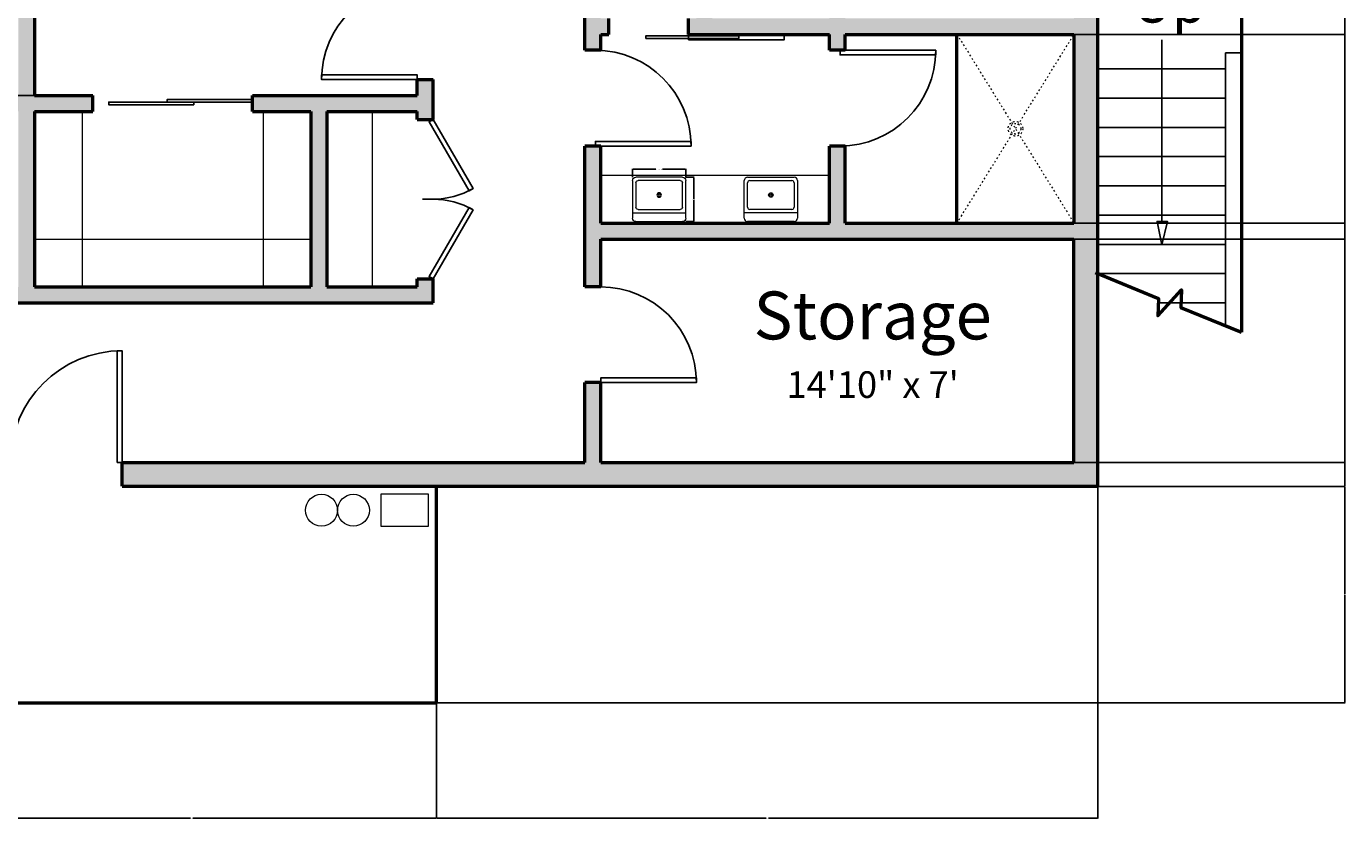
# Model space of a CAD drawing. Units: inches. Extents: x 296 to 2116, y 330 to 1460.
# Tile 8 of 9: x 1620 to 2116, y 779 to 1077. Entities that reach past the tile are written whole.
import ezdxf

# ---------------------------------------------------------------- set-up
doc = ezdxf.new("R2010")
doc.units = ezdxf.units.IN
doc.linetypes.add('ACAD_ISO03W100', pattern=[30, 12, -18])
for name, color, linetype, lineweight in [('A-ANNO-DIMS', 2, 'Continuous', 18), ('A-ANNO-TEXT', 7, 'Continuous', 18), ('A-AREA-IDEN', 7, 'Continuous', 25), ('A-DOOR', 3, 'Continuous', 25), ('A-FLOR-FIXT', 8, 'Continuous', 18), ('A-FLOR-OVHD', 132, 'ACAD_ISO03W100', 18), ('A-FLOR-STRS', 40, 'Continuous', 25), ('A-WALL', 7, 'Continuous', 50), ('A-WALL-PATT', 8, 'Continuous', 13)]:
    doc.layers.add(name, color=color, linetype=linetype, lineweight=lineweight)
doc.styles.add('ATTR', font='romans.shx', dxfattribs={"width": 0.8, "height": 1.075})
doc.styles.get("Standard").update_dxf_attribs({"font": 'arial.ttf'})
doc.dimstyles.get("Standard").update_dxf_attribs({"dimtxt": 0.18, "dimasz": 0.18, "dimexe": 0.18, "dimexo": 0.0625, "dimgap": 0.09, "dimtad": 0, "dimtih": 1, "dimtoh": 1, "dimdec": 4, "dimzin": 0, "dimdsep": 46, "dimtxsty": 'Standard', "dimcen": 0.09, "dimadec": 0, "dimazin": 0, "dimtfac": 1, "dimtdec": 4, "dimtofl": 0, "dimtmove": 0, "dimatfit": 3, "dimfxl": 1, "dimtolj": 1, "dimtzin": 0, "dimarcsym": 0})

# ---------------------------------------------------------------- blocks, each defined once
blk = doc.blocks.new('*U18')
for p, q in [((0, 0), (0, 4)), ((36, 0), (36, 4))]:
    blk.add_line(p, q)
blk.add_lwpolyline([(0, 0), (0, -36), (1.75, -36), (1.75, 0)], close=True)
blk.add_arc((0, 0), 36, 270, 0)
blk = doc.blocks.new('*U19')
for p, q in [((0, 0), (0, -4)), ((36, 0), (36, -4))]:
    blk.add_line(p, q)
blk.add_lwpolyline([(0, 0), (0, 36), (1.75, 36), (1.75, 0)], close=True)
blk.add_arc((0, 0), 36, 0, 90)
blk = doc.blocks.new('*U23')
for p, q in [((-40, 0), (-40, -4)), ((0, 0), (0, -4))]:
    blk.add_line(p, q)
blk.add_lwpolyline([(0, 0), (0, 40), (-1.75, 40), (-1.75, 0)], close=True)
blk.add_arc((0, 0), 40, 90, 180)
blk = doc.blocks.new('*U24')
for p, q in [((0, 0), (0, 4)), ((36, 0), (36, 4))]:
    blk.add_line(p, q)
blk.add_lwpolyline([(0, 0), (0, -36), (1.75, -36), (1.75, 0)], close=True)
blk.add_arc((0, 0), 36, 270, 0)
blk = doc.blocks.new('*U25')
for p, q in [((-36, 0), (-36, 4)), ((0, 0), (0, 4))]:
    blk.add_line(p, q)
blk.add_lwpolyline([(0, 0), (0, -36), (-1.75, -36), (-1.75, 0)], close=True)
blk.add_arc((0, 0), 36, 180, 270)
blk = doc.blocks.new('*U26')
for p, q in [((-30, 0), (-30, 4)), ((0, 0), (0, 4))]:
    blk.add_line(p, q)
blk.add_lwpolyline([(0, 0), (-25.98, -15), (-26.86, -13.48), (-0.88, 1.52)], close=True)
blk.add_arc((0, 0), 30, 180, 210)
blk = doc.blocks.new("24'' Sink Single PV")
blk.add_line((-12.00001, -3.999996), (12, -3.999996))
for points in [[(-10.5, 0), (10.5, 0)], [(-12.00001, -18.499996), (-12.00001, -1.5)], [(-9.5, -5.499996), (9.5, -5.499996)], [(12, -1.5), (12, -18.499996)], [(-10.5, -17.499996), (-10.5, -6.499996)], [(10.5, -6.499996), (10.5, -17.499996)], [(10.5, -19.999996), (-10.5, -19.999996)], [(9.5, -18.499996), (-9.5, -18.499996)]]:
    blk.add_lwpolyline(points)
for radius in [1, 0.5]:
    blk.add_circle((0, -11.999996), radius)
for centre, radius, start, end in [((-10.5, -1.5), 1.5, 90, 180), ((-9.5, -6.499996), 1, 90, 180), ((9.5, -6.499996), 1, 0, 90), ((10.5, -1.5), 1.5, 0, 90), ((-9.5, -17.499996), 1, 180, 270), ((9.5, -17.499996), 1, 270, 0), ((-10.5, -18.499996), 1.5, 180, 270), ((10.5, -18.499996), 1.5, 270, 0)]:
    blk.add_arc(centre, radius, start, end)
at = {"style": 'ATTR', "width": 0.8, "flags": 9}
blk.add_attdef('ESTCODE', (0, 0), '', height=0.0048, dxfattribs=at)
blk = doc.blocks.new('*D37')
at = {"layer": 'A-ANNO-DIMS', "color": 0, "lineweight": -2, "transparency": 16777216}
for p, q in [((1848.18, 1020.25), (1848.18, 1023.37)), ((1848.36, 1023.19), (1856.96, 1023.19)), ((1868, 1023.19), (1859.41, 1023.19)), ((1868.18, 1020.25), (1868.18, 1023.37))]:
    blk.add_line(p, q, dxfattribs=at)
at = {"layer": 'A-ANNO-DIMS', "color": 0, "transparency": 16777216}
for points in [[(1848.36, 1023.22), (1848.36, 1023.16), (1848.18, 1023.19)], [(1868, 1023.22), (1868, 1023.16), (1868.18, 1023.19)]]:
    blk.add_solid(points, dxfattribs=at)
at = {"layer": 'Defpoints', "color": 0, "transparency": 16777216}
for p in [(1868.18, 1023.19), (1848.18, 1020.19), (1868.18, 1020.19)]:
    blk.add_point(p, dxfattribs=at)
at = {"layer": 'A-ANNO-DIMS', "color": 0, "transparency": 16777216, "insert": (1858.18, 1023.19), "char_height": 0.18, "attachment_point": 5}
blk.add_mtext('\\A1;BATH SINK 20 TYP.', dxfattribs=at)
blk = doc.blocks.new('*D38')
at = {"layer": 'A-ANNO-DIMS', "color": 0, "lineweight": -2, "transparency": 16777216}
for p, q in [((1868.25, 1020.19), (1871.36, 1020.19)), ((1871.18, 1020.01), (1871.18, 1012.03)), ((1871.18, 1003.7), (1871.18, 1011.67)), ((1868.25, 1003.52), (1871.36, 1003.52))]:
    blk.add_line(p, q, dxfattribs=at)
at = {"layer": 'A-ANNO-DIMS', "color": 0, "transparency": 16777216}
for points in [[(1871.15, 1020.01), (1871.21, 1020.01), (1871.18, 1020.19)], [(1871.15, 1003.7), (1871.21, 1003.7), (1871.18, 1003.52)]]:
    blk.add_solid(points, dxfattribs=at)
at = {"layer": 'Defpoints', "color": 0, "transparency": 16777216}
for p in [(1868.18, 1020.19), (1868.18, 1003.52), (1871.18, 1003.52)]:
    blk.add_point(p, dxfattribs=at)
at = {"layer": 'A-ANNO-DIMS', "color": 0, "transparency": 16777216, "insert": (1871.18, 1011.85), "char_height": 0.18, "attachment_point": 5}
blk.add_mtext('\\A1;17 TYP.', dxfattribs=at)
blk = doc.blocks.new('*D71')
at = {"layer": 'A-ANNO-DIMS', "color": 0, "lineweight": -2, "transparency": 16777216}
for p, q in [((1590.18, 822.44), (1590.18, 778.97)), ((1774.45, 822.44), (1774.45, 778.97)), ((1590.36, 779.15), (1681.86, 779.15)), ((1774.27, 779.15), (1682.77, 779.15))]:
    blk.add_line(p, q, dxfattribs=at)
at = {"layer": 'A-ANNO-DIMS', "color": 0, "transparency": 16777216}
for points in [[(1590.36, 779.18), (1590.36, 779.12), (1590.18, 779.15)], [(1774.27, 779.18), (1774.27, 779.12), (1774.45, 779.15)]]:
    blk.add_solid(points, dxfattribs=at)
at = {"layer": 'Defpoints', "color": 0, "transparency": 16777216}
for p in [(1590.18, 822.5), (1774.45, 822.5), (1774.45, 779.15)]:
    blk.add_point(p, dxfattribs=at)
at = {"layer": 'A-ANNO-DIMS', "color": 0, "transparency": 16777216, "insert": (1682.31, 779.15), "char_height": 0.18, "attachment_point": 5}
blk.add_mtext('\\A1;184.26', dxfattribs=at)
blk = doc.blocks.new('*D72')
at = {"layer": 'A-ANNO-DIMS', "color": 0, "lineweight": -2, "transparency": 16777216}
for p, q in [((2023.18, 903.89), (2023.18, 778.97)), ((1774.45, 822.44), (1774.45, 778.97)), ((1774.63, 779.15), (1898.35, 779.15)), ((2023, 779.15), (1899.28, 779.15))]:
    blk.add_line(p, q, dxfattribs=at)
at = {"layer": 'A-ANNO-DIMS', "color": 0, "transparency": 16777216}
for points in [[(1774.63, 779.18), (1774.63, 779.12), (1774.45, 779.15)], [(2023, 779.18), (2023, 779.12), (2023.18, 779.15)]]:
    blk.add_solid(points, dxfattribs=at)
at = {"layer": 'Defpoints', "color": 0, "transparency": 16777216}
for p in [(2023.18, 903.95), (1774.45, 822.5), (2023.18, 779.15)]:
    blk.add_point(p, dxfattribs=at)
at = {"layer": 'A-ANNO-DIMS', "color": 0, "transparency": 16777216, "insert": (1898.81, 779.15), "char_height": 0.18, "attachment_point": 5}
blk.add_mtext('\\A1;248.74', dxfattribs=at)
blk = doc.blocks.new('*D73')
at = {"layer": 'A-ANNO-DIMS', "color": 0, "lineweight": -2, "transparency": 16777216}
for p, q in [((2023.25, 903.95), (2116.21, 903.95)), ((2116.03, 903.77), (2116.03, 863.41)), ((2116.03, 822.68), (2116.03, 863.04)), ((1774.51, 822.5), (2116.21, 822.5))]:
    blk.add_line(p, q, dxfattribs=at)
at = {"layer": 'A-ANNO-DIMS', "color": 0, "transparency": 16777216}
for points in [[(2116, 903.77), (2116.06, 903.77), (2116.03, 903.95)], [(2116, 822.68), (2116.06, 822.68), (2116.03, 822.5)]]:
    blk.add_solid(points, dxfattribs=at)
at = {"layer": 'Defpoints', "color": 0, "transparency": 16777216}
for p in [(2023.18, 903.95), (2116.03, 903.95), (1774.45, 822.5)]:
    blk.add_point(p, dxfattribs=at)
at = {"layer": 'A-ANNO-DIMS', "color": 0, "transparency": 16777216, "insert": (2116.03, 863.23), "char_height": 0.18, "attachment_point": 5}
blk.add_mtext('\\A1;81.46', dxfattribs=at)
blk = doc.blocks.new('*D74')
at = {"layer": 'A-ANNO-DIMS', "color": 0, "lineweight": -2, "transparency": 16777216}
for p, q in [((2023.25, 1353.95), (2116.21, 1353.95)), ((2116.03, 1353.77), (2116.03, 1129.14)), ((2116.03, 904.13), (2116.03, 1128.77)), ((2023.25, 903.95), (2116.21, 903.95))]:
    blk.add_line(p, q, dxfattribs=at)
at = {"layer": 'A-ANNO-DIMS', "color": 0, "transparency": 16777216}
for points in [[(2116, 1353.77), (2116.06, 1353.77), (2116.03, 1353.95)], [(2116, 904.13), (2116.06, 904.13), (2116.03, 903.95)]]:
    blk.add_solid(points, dxfattribs=at)
at = {"layer": 'Defpoints', "color": 0, "transparency": 16777216}
for p in [(2023.18, 1353.95), (2116.03, 1353.95), (2023.18, 903.95)]:
    blk.add_point(p, dxfattribs=at)
at = {"layer": 'A-ANNO-DIMS', "color": 0, "transparency": 16777216, "insert": (2116.03, 1128.95), "char_height": 0.18, "attachment_point": 5}
blk.add_mtext('\\A1;450', dxfattribs=at)
blk = doc.blocks.new('*D118')
at = {"layer": 'A-ANNO-DIMS', "color": 0, "lineweight": -2, "transparency": 16777216}
for p, q in [((1623.12, 1210.95), (1276.15, 1210.95)), ((1276.33, 1210.77), (1276.33, 1131.14)), ((1276.33, 1051.13), (1276.33, 1130.77)), ((1623.12, 1050.95), (1276.15, 1050.95))]:
    blk.add_line(p, q, dxfattribs=at)
at = {"layer": 'A-ANNO-DIMS', "color": 0, "transparency": 16777216}
for points in [[(1276.3, 1210.77), (1276.36, 1210.77), (1276.33, 1210.95)], [(1276.3, 1051.13), (1276.36, 1051.13), (1276.33, 1050.95)]]:
    blk.add_solid(points, dxfattribs=at)
at = {"layer": 'Defpoints', "color": 0, "transparency": 16777216}
for p in [(1276.33, 1210.95), (1623.18, 1210.95), (1623.18, 1050.95)]:
    blk.add_point(p, dxfattribs=at)
at = {"layer": 'A-ANNO-DIMS', "color": 0, "transparency": 16777216, "insert": (1276.33, 1130.95), "char_height": 0.18, "attachment_point": 5}
blk.add_mtext('\\A1;160.00', dxfattribs=at)
blk = doc.blocks.new('*D122')
at = {"layer": 'A-ANNO-DIMS', "color": 0, "lineweight": -2, "transparency": 16777216}
for p, q in [((2014.25, 996.95), (2116.21, 996.95)), ((2116.03, 996.77), (2116.03, 955.14)), ((2116.03, 913.13), (2116.03, 954.77)), ((2014.25, 912.95), (2116.21, 912.95))]:
    blk.add_line(p, q, dxfattribs=at)
at = {"layer": 'A-ANNO-DIMS', "color": 0, "transparency": 16777216}
for points in [[(2116, 996.77), (2116.06, 996.77), (2116.03, 996.95)], [(2116, 913.13), (2116.06, 913.13), (2116.03, 912.95)]]:
    blk.add_solid(points, dxfattribs=at)
at = {"layer": 'Defpoints', "color": 0, "transparency": 16777216}
for p in [(2014.18, 996.95), (2116.03, 996.95), (2014.18, 912.95)]:
    blk.add_point(p, dxfattribs=at)
at = {"layer": 'A-ANNO-DIMS', "color": 0, "transparency": 16777216, "insert": (2116.03, 954.95), "char_height": 0.18, "attachment_point": 5}
blk.add_mtext('\\A1;84.00', dxfattribs=at)
blk = doc.blocks.new('*D123')
at = {"layer": 'A-ANNO-DIMS', "color": 0, "lineweight": -2, "transparency": 16777216}
for p, q in [((2014.25, 1073.95), (2116.21, 1073.95)), ((2116.03, 1073.77), (2116.03, 1038.64)), ((2116.03, 1003.13), (2116.03, 1038.27)), ((2014.25, 1002.95), (2116.21, 1002.95))]:
    blk.add_line(p, q, dxfattribs=at)
at = {"layer": 'A-ANNO-DIMS', "color": 0, "transparency": 16777216}
for points in [[(2116, 1073.77), (2116.06, 1073.77), (2116.03, 1073.95)], [(2116, 1003.13), (2116.06, 1003.13), (2116.03, 1002.95)]]:
    blk.add_solid(points, dxfattribs=at)
at = {"layer": 'Defpoints', "color": 0, "transparency": 16777216}
for p in [(2014.18, 1073.95), (2116.03, 1073.95), (2014.18, 1002.95)]:
    blk.add_point(p, dxfattribs=at)
at = {"layer": 'A-ANNO-DIMS', "color": 0, "transparency": 16777216, "insert": (2116.03, 1038.45), "char_height": 0.18, "attachment_point": 5}
blk.add_mtext('\\A1;71.00', dxfattribs=at)

msp = doc.modelspace()

# ---------------------------------------------------------------- hatches: boundary and pattern name
at = {"layer": 'A-WALL-PATT'}
h = msp.add_hatch(color=256, dxfattribs=at)
h.dxf.hatch_style = 1
h.paths.add_polyline_path([(1321.1832, 1353.9541), (1315.1832, 1353.9541), (1315.1832, 1347.9541), (1321.1832, 1347.9541)])
h.paths.add_polyline_path([(1496.1832, 1353.9541), (1490.1832, 1353.9541), (1490.1832, 1347.9541), (1496.1832, 1347.9541)])
h.paths.add_polyline_path([(1396.1832, 1189.9541), (1392.1832, 1189.9541), (1392.1832, 1180.9541), (1396.1832, 1180.9541)])
h.paths.add_polyline_path([(1436.1832, 1189.9541), (1432.1832, 1189.9541), (1432.1832, 1180.9541), (1436.1832, 1180.9541), (1436.1832, 1184.9541)])
h.paths.add_polyline_path([(1356.1832, 1189.9541), (1318.1832, 1189.9541), (1318.1832, 1138.9541), (1322.6832, 1138.9541), (1322.6832, 1144.9541), (1327.1832, 1144.9541), (1327.1832, 1180.9541), (1356.1832, 1180.9541)])
h.paths.add_polyline_path([(1499.1832, 1210.9541), (1523.1832, 1210.9541), (1523.1832, 1219.9541), (1490.1832, 1219.9541), (1490.1832, 1189.9541), (1472.1832, 1189.9541), (1472.1832, 1180.9541), (1499.1832, 1180.9541)])
h.paths.add_polyline_path([(1635.1832, 1219.9541), (1599.1832, 1219.9541), (1599.1832, 1210.9541), (1617.1832, 1210.9541), (1617.1832, 1050.9541), (1581.1832, 1050.9541), (1581.1832, 1041.9541), (1587.1832, 1041.9541), (1587.1832, 1044.9541), (1617.1832, 1044.9541), (1617.1832, 978.9541), (1587.1832, 978.9541), (1587.1832, 981.9541), (1581.1832, 981.9541), (1581.1832, 966.9541), (1587.1832, 966.9541), (1587.1832, 972.9541), (1773.1832, 972.9541), (1773.1832, 981.9541), (1767.1832, 981.9541), (1767.1832, 978.9541), (1733.1832, 978.9541), (1733.1832, 1044.9541), (1767.1832, 1044.9541), (1767.1832, 1041.9541), (1773.1832, 1041.9541), (1773.1832, 1056.9541), (1767.1832, 1056.9541), (1767.1832, 1050.9541), (1705.1832, 1050.9541), (1705.1832, 1044.9541), (1727.1832, 1044.9541), (1727.1832, 978.9541), (1623.1832, 978.9541), (1623.1832, 1044.9541), (1645.1832, 1044.9541), (1645.1832, 1050.9541), (1623.1832, 1050.9541), (1623.1832, 1210.9541), (1635.1832, 1210.9541)])
h.paths.add_polyline_path([(1773.1832, 1250.9541), (1767.1832, 1250.9541), (1767.1832, 1216.9541), (1719.1832, 1216.9541), (1719.1832, 1344.9541), (1767.1832, 1344.9541), (1767.1832, 1310.9541), (1773.1832, 1310.9541), (1773.1832, 1344.9541), (1779.1832, 1344.9541), (1779.1832, 1353.9541), (1710.1832, 1353.9541), (1710.1832, 1219.9541), (1699.1832, 1219.9541), (1699.1832, 1210.9541), (1767.1832, 1210.9541), (1767.1832, 1092.9541), (1773.1832, 1092.9541), (1773.1832, 1114.9541), (1780.6832, 1114.9541), (1780.6832, 1120.9541), (1773.1832, 1120.9541)])
h.paths.add_polyline_path([(1360.1832, 899.9541), (1327.1832, 899.9541), (1327.1832, 918.4541), (1322.6832, 918.4541), (1322.6832, 921.4541), (1318.1832, 921.4541), (1318.1832, 890.9541), (1351.1832, 890.9541), (1351.1832, 817.9991), (1590.1832, 817.9991), (1590.1832, 903.9541), (1614.1832, 903.9541), (1614.1832, 912.9541), (1587.1832, 912.9541), (1587.1832, 918.9541), (1581.1832, 918.9541), (1581.1832, 880.9991), (1420.1332, 880.9991), (1420.1332, 918.9541), (1415.9332, 918.9541), (1414.1332, 918.9541), (1414.1332, 874.9991), (1581.1832, 874.9991), (1581.1832, 826.9991), (1360.1832, 826.9991)])
h.paths.add_polyline_path([(1327.1832, 1056.9541), (1322.6832, 1056.9541), (1322.6832, 1062.9541), (1318.1832, 1062.9541), (1318.1832, 951.4541), (1322.6832, 951.4541), (1322.6832, 954.4541), (1327.1832, 954.4541), (1327.1832, 972.9541), (1414.1332, 972.9541), (1414.1332, 960.9541), (1420.1332, 960.9541), (1420.1332, 978.9541), (1327.1832, 978.9541)])
h.paths.add_polyline_path([(2023.1832, 1106.4482), (2018.6832, 1106.4482), (2018.6832, 1103.4482), (2014.1832, 1103.4482), (2014.1832, 1079.9541), (1928.1832, 1079.9541), (1928.1832, 1082.9541), (1922.1832, 1082.9541), (1922.1832, 1079.9541), (1878.1832, 1079.9541), (1878.1832, 1150.9541), (1881.1832, 1150.9541), (1881.1832, 1154.9541), (1881.1832, 1156.9541), (1830.1832, 1156.9541), (1830.1832, 1120.9541), (1822.6832, 1120.9541), (1822.6832, 1116.7541), (1822.6832, 1114.9541), (1830.1832, 1114.9541), (1830.1832, 1067.9541), (1834.1832, 1067.9541), (1836.1832, 1067.9541), (1836.1832, 1073.9541), (1839.1832, 1073.9541), (1839.1832, 1079.9541), (1836.1832, 1079.9541), (1836.1832, 1150.9541), (1872.1832, 1150.9541), (1872.1832, 1079.9541), (1869.1832, 1079.9541), (1869.1832, 1073.9541), (1905.1832, 1073.9541), (1922.1832, 1073.9541), (1922.1832, 1067.9541), (1926.1832, 1067.9541), (1928.1832, 1067.9541), (1928.1832, 1073.9541), (2014.1832, 1073.9541), (2014.1832, 1002.9541), (1970.1832, 1002.9541), (1928.1832, 1002.9541), (1928.1832, 1031.9541), (1922.1832, 1031.9541), (1922.1832, 1002.9541), (1836.1832, 1002.9541), (1836.1832, 1031.9541), (1834.1832, 1031.9541), (1830.1832, 1031.9541), (1830.1832, 978.9541), (1836.1832, 978.9541), (1836.1832, 996.9541), (2014.1832, 996.9541), (2014.1832, 912.9541), (1836.1832, 912.9541), (1836.1832, 942.9541), (1832.1832, 942.9541), (1830.1832, 942.9541), (1830.1832, 912.9541), (1656.1832, 912.9541), (1656.1832, 908.7541), (1656.1832, 903.9541), (2023.1832, 903.9541)])
h.paths.add_polyline_path([(2023.1832, 1165.9541), (1958.1832, 1165.9541), (1958.1832, 1156.9541), (2014.1832, 1156.9541), (2014.1832, 1139.4482), (2018.6832, 1139.4482), (2018.6832, 1136.4482), (2023.1832, 1136.4482), (2023.1832, 1159.9541)])
h.paths.add_polyline_path([(1934.1832, 1165.9541), (1928.1832, 1165.9541), (1928.1832, 1186.9541), (1923.6832, 1186.9541), (1923.6832, 1183.9541), (1919.1832, 1183.9541), (1919.1832, 1156.9541), (1911.1832, 1156.9541), (1911.1832, 1150.9541), (1922.1832, 1150.9541), (1922.1832, 1147.9541), (1928.1832, 1147.9541), (1928.1832, 1156.9541), (1934.1832, 1156.9541)])
h.paths.add_polyline_path([(1928.1832, 1293.9541), (1923.6832, 1293.9541), (1923.6832, 1290.9541), (1919.1832, 1290.9541), (1919.1832, 1219.9541), (1923.6832, 1219.9541), (1923.6832, 1216.9541), (1928.1832, 1216.9541)])
h.paths.add_polyline_path([(1928.1832, 1353.9541), (1854.1832, 1353.9541), (1854.1832, 1344.9541), (1919.1832, 1344.9541), (1919.1832, 1326.9541), (1923.6832, 1326.9541), (1923.6832, 1323.9541), (1928.1832, 1323.9541)])
h.paths.add_polyline_path([(1818.1832, 1353.9541), (1815.1832, 1353.9541), (1815.1832, 1344.9541), (1818.1832, 1344.9541)])
h.paths.add_polyline_path([(1563.1832, 1219.9541), (1559.1832, 1219.9541), (1559.1832, 1210.9541), (1563.1832, 1210.9541)])
h.paths.add_polyline_path([(1669.1832, 1219.9541), (1665.1832, 1219.9541), (1665.1832, 1210.9541), (1669.1832, 1210.9541)])
h.paths.add_polyline_path([(1322.6832, 1102.9541), (1318.1832, 1102.9541), (1318.1832, 1098.9541), (1322.6832, 1098.9541)])

# ---------------------------------------------------------------- linework, layer by layer
at = {"layer": 'A-DOOR'}
for points in [[(1853.1832, 1072.4541), (1888.1832, 1072.4541), (1888.1832, 1073.4541), (1853.1832, 1073.4541)], [(1869.1832, 1071.9541), (1905.1832, 1071.9541), (1905.1832, 1073.9541), (1869.1832, 1073.9541)], [(1683.1832, 1047.4541), (1683.1832, 1048.4541), (1651.1832, 1048.4541), (1651.1832, 1047.4541)], [(1705.1832, 1048.4541), (1705.1832, 1049.4541), (1673.1832, 1049.4541), (1673.1832, 1048.4541)]]:
    msp.add_lwpolyline(points, close=True, dxfattribs=at)
at = {"layer": 'A-FLOR-FIXT'}
for p, q in [((1641.1832, 1044.9541), (1641.1832, 978.9541)), ((1709.1832, 1044.9541), (1709.1832, 978.9541)), ((1750.1832, 1044.9541), (1750.1832, 978.9541)), ((1836.1832, 1020.9541), (1922.1832, 1020.9541)), ((1623.1832, 996.9541), (1727.1832, 996.9541))]:
    msp.add_line(p, q, dxfattribs=at)
msp.add_lwpolyline([(1753.4453, 888.9541), (1771.4453, 888.9541), (1771.4453, 900.9541), (1753.4453, 900.9541)], close=True, dxfattribs=at)
for centre in [(1731.1691, 894.9541), (1743.1691, 894.9541)]:
    msp.add_circle(centre, 6, dxfattribs=at)
at = {"layer": 'A-FLOR-OVHD', "ltscale": 0.05}
for p, q in [((1970.1832, 1002.9541), (2014.1832, 1073.9541)), ((1970.1832, 1073.9541), (2014.1832, 1002.9541))]:
    msp.add_line(p, q, dxfattribs=at)
msp.add_lwpolyline([(2014.1832, 1073.9541), (1970.1832, 1073.9541), (1970.1832, 1002.9541), (2014.1832, 1002.9541)], close=True, dxfattribs=at)
for radius in [2.75, 2]:
    msp.add_circle((1992.1832, 1038.4541), radius, dxfattribs=at)
at = {"layer": 'A-FLOR-STRS'}
for p, q in [((2071.1832, 964.3985), (2071.1832, 1066.9541)), ((2071.1832, 1066.9541), (2077.1832, 1066.9541)), ((2071.1832, 1060.9541), (2023.1832, 1060.9541)), ((2071.1832, 1049.9541), (2023.1832, 1049.9541)), ((2071.1832, 1038.9541), (2023.1832, 1038.9541)), ((2071.1832, 1027.9541), (2023.1832, 1027.9541)), ((2071.1832, 1016.9541), (2023.1832, 1016.9541)), ((2071.1832, 1005.9541), (2023.1832, 1005.9541)), ((2071.1832, 994.9541), (2023.1832, 994.9541)), ((2071.1832, 983.9541), (2023.1832, 983.9541)), ((2071.1832, 972.9541), (2045.9516, 972.9541))]:
    msp.add_line(p, q, dxfattribs=at)
msp.add_lwpolyline([(2047.1832, 1071.9541), (2047.1832, 1003.6135)], dxfattribs=at)
msp.add_lwpolyline([(2047.1832, 994.7456), (2049.3282, 1003.6135), (2045.435, 1003.6135)], close=True, dxfattribs=at)
at = {"layer": 'A-WALL'}
for p, q in [((2077.1832, 1407.9541), (2077.1832, 961.9541)), ((1623.1832, 1210.9541), (1623.1832, 1050.9541)), ((1830.1832, 1067.9541), (1830.1832, 1114.9541)), ((2023.1832, 903.9541), (2023.1832, 1108.9541)), ((1839.1832, 1073.9541), (1839.1832, 1079.9541)), ((1869.1832, 1073.9541), (1869.1832, 1079.9541)), ((1836.1832, 1073.9541), (1839.1832, 1073.9541)), ((1836.1832, 1067.9541), (1836.1832, 1073.9541)), ((1869.1832, 1073.9541), (1922.1832, 1073.9541)), ((1922.1832, 1067.9541), (1922.1832, 1073.9541)), ((1928.1832, 1073.9541), (2014.1832, 1073.9541)), ((1928.1832, 1067.9541), (1928.1832, 1073.9541)), ((1970.1832, 1002.9541), (1970.1832, 1073.9541)), ((2014.1832, 1073.9541), (2014.1832, 1002.9541)), ((1836.1832, 1067.9541), (1830.1832, 1067.9541)), ((1928.1832, 1067.9541), (1922.1832, 1067.9541)), ((1767.1832, 1050.9541), (1767.1832, 1056.9541)), ((1767.1832, 1056.9541), (1773.1832, 1056.9541)), ((1773.1832, 1041.9541), (1773.1832, 1056.9541)), ((1623.1832, 1050.9541), (1645.1832, 1050.9541)), ((1645.1832, 1044.9541), (1645.1832, 1050.9541)), ((1705.1832, 1044.9541), (1705.1832, 1050.9541)), ((1705.1832, 1050.9541), (1767.1832, 1050.9541)), ((1623.1832, 1044.9541), (1623.1832, 978.9541)), ((1623.1832, 1044.9541), (1645.1832, 1044.9541)), ((1705.1832, 1044.9541), (1727.1832, 1044.9541)), ((1727.1832, 1044.9541), (1727.1832, 978.9541)), ((1733.1832, 1044.9541), (1733.1832, 978.9541)), ((1733.1832, 1044.9541), (1767.1832, 1044.9541)), ((1767.1832, 1041.9541), (1767.1832, 1044.9541)), ((1767.1832, 1041.9541), (1773.1832, 1041.9541)), ((1830.1832, 978.9541), (1830.1832, 1031.9541)), ((1836.1832, 1031.9541), (1830.1832, 1031.9541)), ((1836.1832, 1002.9541), (1836.1832, 1031.9541)), ((1922.1832, 1002.9541), (1922.1832, 1031.9541)), ((1928.1832, 1031.9541), (1922.1832, 1031.9541)), ((1928.1832, 1002.9541), (1928.1832, 1031.9541)), ((1836.1832, 1002.9541), (1922.1832, 1002.9541)), ((1928.1832, 1002.9541), (2014.1832, 1002.9541)), ((1836.1832, 996.9541), (2014.1832, 996.9541)), ((1836.1832, 978.9541), (1836.1832, 996.9541)), ((2014.1832, 912.9541), (2014.1832, 996.9541)), ((1623.1832, 978.9541), (1727.1832, 978.9541)), ((1733.1832, 978.9541), (1767.1832, 978.9541)), ((1767.1832, 978.9541), (1767.1832, 981.9541)), ((1767.1832, 981.9541), (1773.1832, 981.9541)), ((1773.1832, 972.9541), (1773.1832, 981.9541)), ((1836.1832, 978.9541), (1830.1832, 978.9541)), ((1587.1832, 972.9541), (1773.1832, 972.9541)), ((1830.1832, 912.9541), (1830.1832, 942.9541)), ((1836.1832, 942.9541), (1830.1832, 942.9541)), ((1836.1832, 912.9541), (1836.1832, 942.9541)), ((1656.1832, 903.9541), (1656.1832, 912.9541)), ((1656.1832, 912.9541), (1830.1832, 912.9541)), ((1836.1832, 912.9541), (2014.1832, 912.9541)), ((1656.1832, 903.9541), (2023.1832, 903.9541)), ((1774.4453, 822.4991), (1774.4453, 903.9541)), ((1590.1832, 822.4991), (1774.4453, 822.4991))]:
    msp.add_line(p, q, dxfattribs=at)
msp.add_lwpolyline([(2022.2571, 984.3314), (2046.0158, 974.6519), (2045.7671, 968.0781), (2054.5993, 977.8301), (2054.3506, 971.2563), (2077.1832, 961.9541)], dxfattribs=at)

# ---------------------------------------------------------------- block references
at = {"layer": 'A-DOOR'}
for name, p, rotation in [('*U19', (1767.1832, 1056.9541), 89.99999999999969), ('*U24', (1834.1832, 1031.9541), 89.99999999999969), ('*U25', (1926.1832, 1067.9541), 89.99999999999969), ('*U26', (1773.1832, 1041.9541), 90), ('*U18', (1836.1832, 942.9541), 89.99999999999969)]:
    msp.add_blockref(name, p, dxfattribs=dict(at, rotation=rotation))
at = {"layer": 'A-DOOR', "xscale": -1, "rotation": 90}
msp.add_blockref('*U26', (1773.1832, 981.9541), dxfattribs=at)
at = {"layer": 'A-DOOR', "xscale": 1.05, "yscale": 1.05, "zscale": 1.05}
msp.add_blockref('*U23', (1656.1832, 912.9541), dxfattribs=at)
at = {"layer": 'A-FLOR-FIXT', "yscale": 0.8333413357028808, "zscale": 0.8333413357028808, "rotation": 180}
for p, xscale in [((1858.1832, 1003.5216), -0.8333413357028808), ((1900.1832, 1003.5216), 0.8333413357028808)]:
    msp.add_blockref("24'' Sink Single PV", p, dxfattribs=dict(at, xscale=xscale))

# ---------------------------------------------------------------- texts
at = {"layer": 'A-ANNO-TEXT', "insert": (2036.3028, 1093.3887), "char_height": 15, "attachment_point": 1}
msp.add_mtext_dynamic_manual_height_columns('{\\fArial|b1|i0|c0|p34;Up}', width=22.506546, gutter_width=12.5, heights=[0], dxfattribs=at)
at = {"layer": 'A-AREA-IDEN', "insert": (1889.0607, 977.2249), "char_height": 24, "attachment_point": 1}
msp.add_mtext_dynamic_manual_height_columns('\\pxqc;{\\fArial|b1|i0|c0|p34;\\H0.75x;Storage\\P\\fArial|b0|i0|c0|p34;\\H0.55556x;14\'10" x 7\'}', width=98.796099, gutter_width=12.5, heights=[0], dxfattribs=at)

# ---------------------------------------------------------------- dimensions: what is measured, and where the dimension line sits
at = {"layer": 'A-ANNO-DIMS'}
for base, p1, p2, override, picture, middle in [((2116.0332, 1353.9541), (2023.1832, 903.9541), (2023.1832, 1353.9541), {"dimdec": 0, "dimlfac": 1, "dimrnd": 0, "dimzin": 0, "dimdsep": 46, "dimlunit": 2}, '*D74', (2116.0332, 1128.9541)), ((1276.3332, 1210.9541), (1623.1832, 1050.9541), (1623.1832, 1210.9541), {"dimdec": 2, "dimlfac": 1, "dimrnd": 0, "dimzin": 0, "dimdsep": 46, "dimlunit": 2}, '*D118', (1276.3332, 1130.9541)), ((2116.0332, 1073.9541), (2014.1832, 1002.9541), (2014.1832, 1073.9541), {"dimdec": 2, "dimlfac": 1, "dimrnd": 0, "dimzin": 0, "dimdsep": 46, "dimlunit": 2}, '*D123', (2116.0332, 1038.4541)), ((2116.0332, 996.9541), (2014.1832, 912.9541), (2014.1832, 996.9541), {"dimdec": 2, "dimlfac": 1, "dimrnd": 0, "dimzin": 0, "dimdsep": 46, "dimlunit": 2}, '*D122', (2116.0332, 954.9541)), ((2116.03322, 903.9541), (1774.44529, 822.49909), (2023.18322, 903.9541), {"dimdec": 2, "dimlfac": 1, "dimrnd": 0, "dimzin": 0, "dimdsep": 46, "dimlunit": 2}, '*D73', (2116.03322, 863.22659))]:
    dim = msp.add_linear_dim(base=base, p1=p1, p2=p2, angle=90, dimstyle='Standard', override=override, dxfattribs=at)
    dim.commit()
    dim.dimension.update_dxf_attribs({"geometry": picture, "text_midpoint": middle})
dim = msp.add_linear_dim(base=(1868.1833, 1023.1884), p1=(1848.1831, 1020.1884), p2=(1868.1833, 1020.1884), text='BATH SINK <> TYP.', dimstyle='Standard', override={"dimdec": 0, "dimrnd": 0, "dimzin": 0, "dimlunit": 2}, dxfattribs=at)
dim.commit()
dim.dimension.update_dxf_attribs({"geometry": '*D37', "text_midpoint": (1858.1832, 1023.1884)})
dim = msp.add_linear_dim(base=(1871.1833, 1003.5176), p1=(1868.1833, 1020.1884), p2=(1868.1833, 1003.5176), angle=270, text='<> TYP.', dimstyle='Standard', override={"dimdec": 0, "dimrnd": 0, "dimzin": 0, "dimlunit": 2}, dxfattribs=at)
dim.commit()
dim.dimension.update_dxf_attribs({"geometry": '*D38', "text_midpoint": (1871.1833, 1011.853)})
for base, p1, p2, picture, middle in [((2023.1832, 779.1491), (1774.4453, 822.4991), (2023.1832, 903.9541), '*D72', (1898.8143, 779.1491)), ((1774.4453, 779.1491), (1590.1832, 822.4991), (1774.4453, 822.4991), '*D71', (1682.3143, 779.1491))]:
    dim = msp.add_linear_dim(base=base, p1=p1, p2=p2, dimstyle='Standard', override={"dimdec": 2, "dimlfac": 1, "dimrnd": 0, "dimzin": 0, "dimdsep": 46, "dimlunit": 2}, dxfattribs=at)
    dim.commit()
    dim.dimension.update_dxf_attribs({"geometry": picture, "text_midpoint": middle})

doc.saveas('drawing.dxf')
